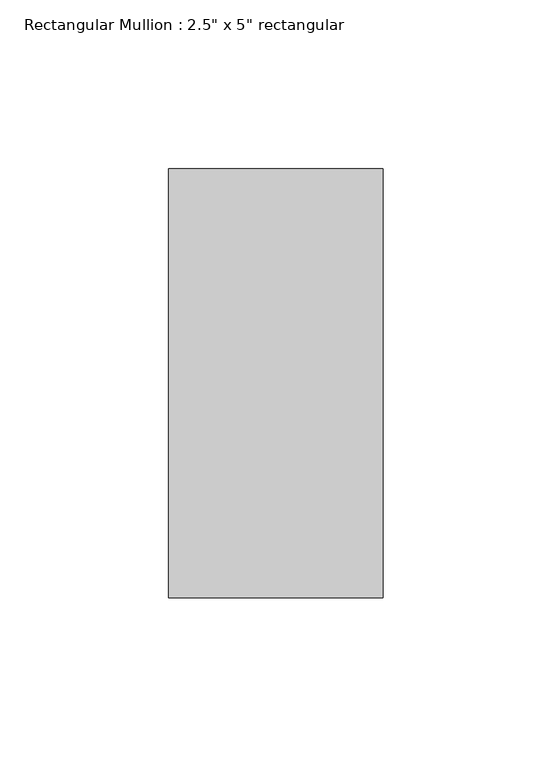
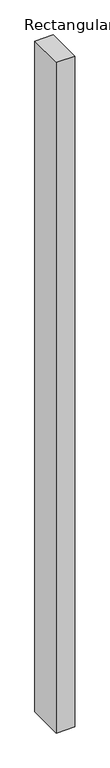
"""IFC4 building model written with IfcOpenShell, lengths in millimetres: member geometry."""

from ifc_helpers import new_model, si_unit, frame, origin, place, context, project, spatial, polyline, outline, extrude, source, transform, mapped, element, save


def member_e878716d(model_context):
    return source(origin(), model_context, "Body", "SweptSolid", [
        extrude(outline(polyline([(0.0, 63.5), (0.0, -63.5), (-63.5, -63.5), (-63.5, 63.5), (0.0, 63.5)])), frame((0.0, 0.0, -2445.7520936), z_axis=(0.0, 0.0, 1.0), x_axis=(1.0, 0.0, 0.0)), (0.0, 0.0, 1.0), 2445.7520936),
    ])


if __name__ == "__main__":
    model = new_model("IFC4")
    model_context = context("Model", 3, world=origin())
    ifc_project = project(units=[si_unit("LENGTHUNIT", "METRE", prefix="MILLI")], contexts=[model_context])
    site = spatial("IfcSite", under=ifc_project)
    building = spatial("IfcBuilding", under=site)
    placement = place(None, origin())
    member_shape = member_e878716d(model_context)
    element("IfcMember", 1, ObjectType="Rectangular Mullion : 2.5\" x 5\" rectangular", at=placement, inside=building, context=model_context, shape_type="MappedRepresentation", body=[
        mapped(member_shape, transform((0.0, 0.0, 0.0), x_axis=(1.0, 0.0, 0.0), y_axis=(0.0, 1.0, 0.0), z_axis=(0.0, 0.0, 1.0))),
    ])
    save(model, "model.ifc")

# Revit data of these elements
# Type "Rectangular Mullion : 2.5\" x 5\" rectangular"
#   built-in parameter 1007304 = 0.416667 (stored number, unit not read)
#   built-in parameter 1007301 = 0.104167 (stored number, unit not read)
#   built-in parameter 1007300 = 0.104167 (stored number, unit not read)
# Element 1 (IfcMember, "Rectangular Mullion : 2.5\" x 5\" rectangular")
#   Materials on its faces: "Aluminum"
# Materials
#   "Aluminum": class "Metal", colour RGB 247 247 247, transparency 0, Description = "Aluminum 6061", Cost = 0
